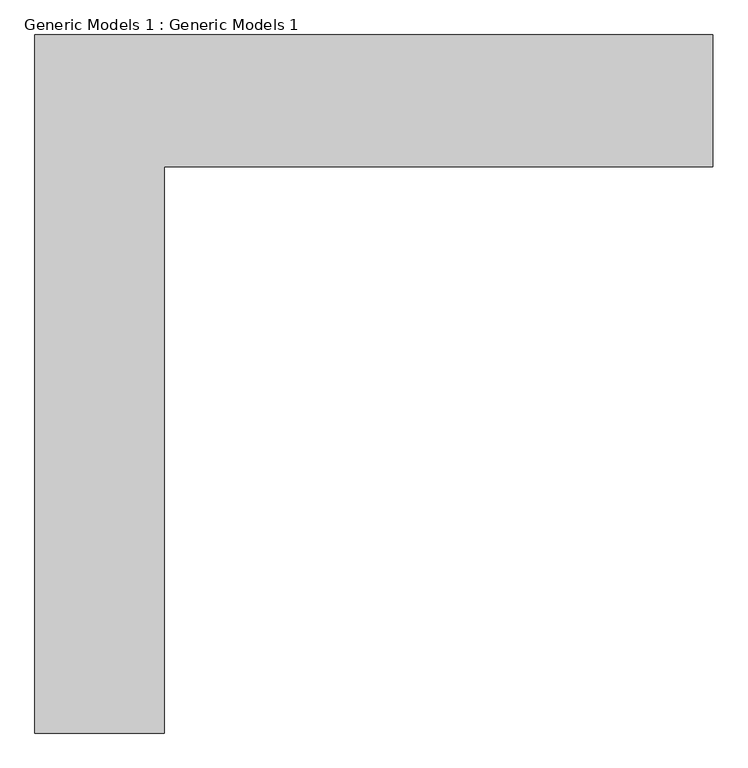
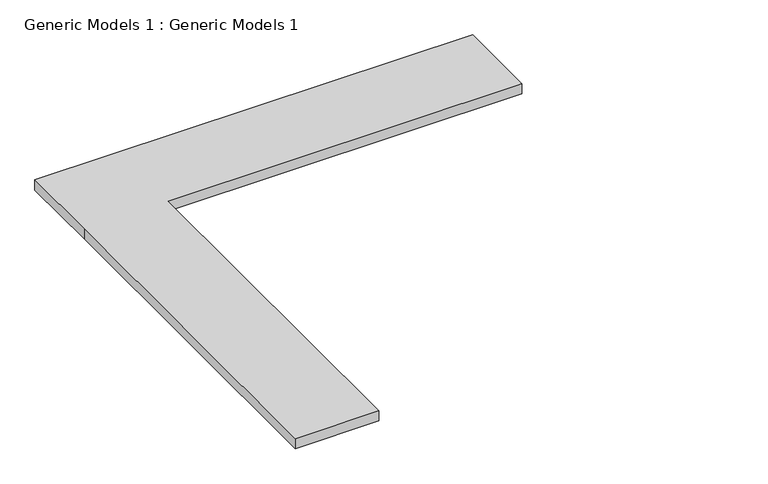
"""IFC4 building model written with IfcOpenShell, lengths in millimetres: proxy geometry, Generic Models 1 : Generic Models 1."""

from ifc_helpers import new_model, si_unit, frame, origin, place, context, project, spatial, polyline, outline, extrude, source, transform, mapped, element, save


def generic_models_1_generic_models_1_ec2a76fc(model_context):
    return source(origin(), model_context, "Body", "SweptSolid", [
        extrude(outline(polyline([(1817.9775609, 10537.8250769), (1817.9775609, 7935.4853898), (1223.7679225, 7935.4853898), (1223.7679225, 10537.8250769), (1223.7679225, 11143.4972041), (4339.2756751, 11143.4972041), (4339.2756751, 10537.8250769), (1817.9775609, 10537.8250769)])), frame((0.0, 0.0, 1219.2), z_axis=(0.0, 0.0, 1.0), x_axis=(1.0, 0.0, 0.0)), (0.0, 0.0, 1.0), 76.2),
    ])


if __name__ == "__main__":
    model = new_model("IFC4")
    model_context = context("Model", 3, world=origin())
    ifc_project = project(units=[si_unit("LENGTHUNIT", "METRE", prefix="MILLI")], contexts=[model_context])
    site = spatial("IfcSite", under=ifc_project)
    building = spatial("IfcBuilding", under=site)
    placement = place(None, origin())
    generic_models_1_generic_models_1_shape = generic_models_1_generic_models_1_ec2a76fc(model_context)
    element("IfcBuildingElementProxy", 1, Name="Generic Models 1 : Generic Models 1", ObjectType="Generic Models 1 : Generic Models 1", at=placement, inside=building, context=model_context, shape_type="MappedRepresentation", body=[
        mapped(generic_models_1_generic_models_1_shape, transform((0.0, 0.0, 0.0), x_axis=(1.0, 0.0, 0.0), y_axis=(0.0, 1.0, 0.0), z_axis=(0.0, 0.0, 1.0))),
    ])
    save(model, "model.ifc")

# Revit data of these elements
# Element 1 (IfcBuildingElementProxy, "Generic Models 1 : Generic Models 1")
#   Materials on its faces: "Cherry"
# Materials
#   "Cherry": class "Wood", colour RGB 226 177 128, transparency 0, Description = "Prunus Serotina", Cost = 0
